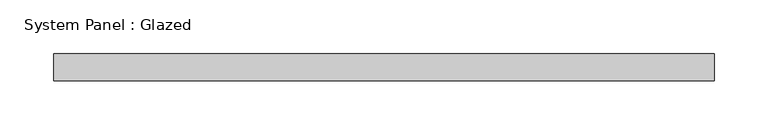
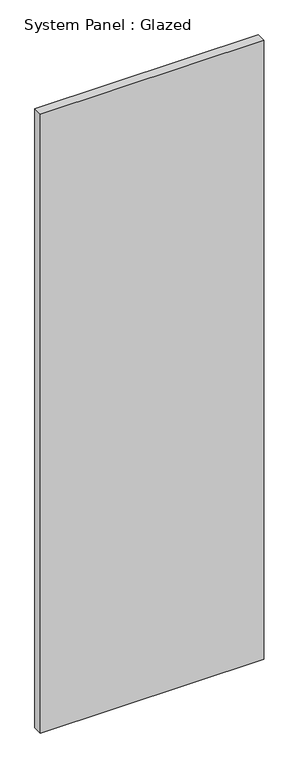
"""IFC4 building model written with IfcOpenShell, lengths in millimetres: plate geometry, System Panel : Glazed."""

from ifc_helpers import new_model, si_unit, origin, origin_with_axes, place, context, project, spatial, polyline, outline, extrude, source, transform, mapped, element, save


def system_panel_glazed_1c0d1104(model_context):
    return source(origin(), model_context, "Body", "SweptSolid", [
        extrude(outline(polyline([(307.975, 19.05), (-307.975, 19.05), (-307.975, 44.45), (307.975, 44.45), (307.975, 19.05)])), origin_with_axes(), (0.0, 0.0, 1.0), 1804.193737),
    ])


if __name__ == "__main__":
    model = new_model("IFC4")
    model_context = context("Model", 3, world=origin())
    ifc_project = project(units=[si_unit("LENGTHUNIT", "METRE", prefix="MILLI")], contexts=[model_context])
    site = spatial("IfcSite", under=ifc_project)
    building = spatial("IfcBuilding", under=site)
    placement = place(None, origin())
    system_panel_glazed_shape = system_panel_glazed_1c0d1104(model_context)
    element("IfcPlate", 1, ObjectType="System Panel : Glazed", at=placement, inside=building, context=model_context, shape_type="MappedRepresentation", body=[
        mapped(system_panel_glazed_shape, transform((0.0, 0.0, 0.0), x_axis=(1.0, 0.0, 0.0), y_axis=(0.0, 1.0, 0.0), z_axis=(0.0, 0.0, 1.0))),
    ])
    save(model, "model.ifc")

# Revit data of these elements
# Type "System Panel : Glazed"
#   Construction Type Id = "GSP4R"
#   Analytic Construction = "1/8 in Pilkington single glazing"
#   Visual Light Transmittance = 0.9
#   Solar Heat Gain Coefficient = 0.86
#   Heat Transfer Coefficient (U) = 1.18115 BTU/(h·ft²·°F)
#   Define Thermal Properties by = 1
# Element 1 (IfcPlate, "System Panel : Glazed")
#   Materials on its faces: "Glass"
# Materials
#   "Glass": class "Glass", colour RGB 0 128 192, transparency 0.75, Description = "Soda Lime Glass", Cost = 0
